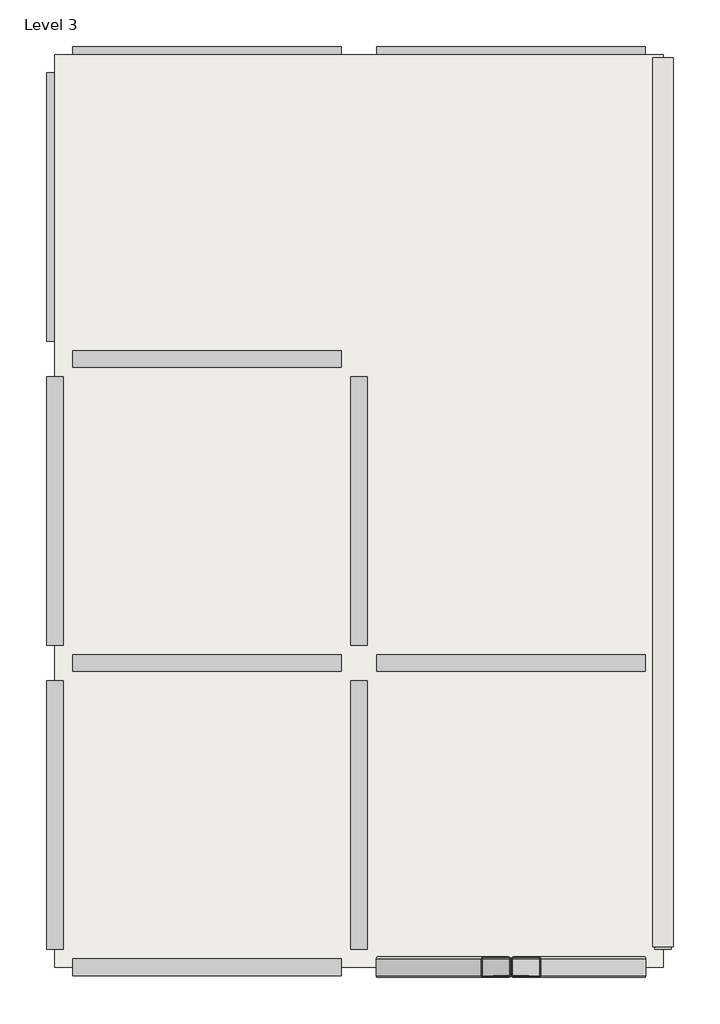
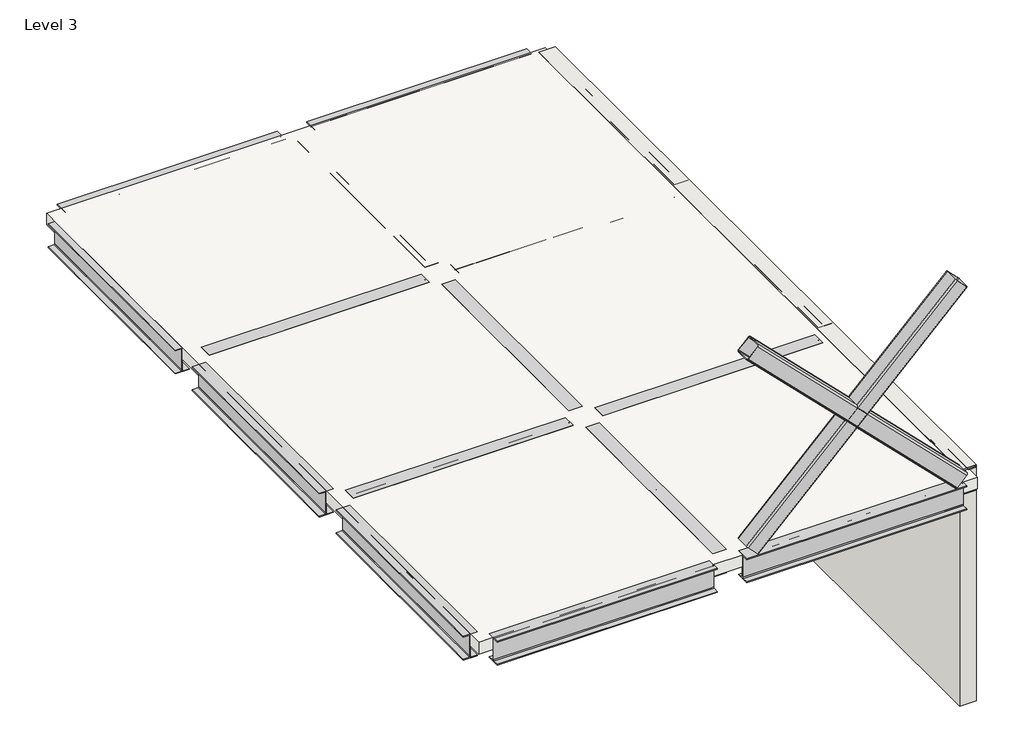
# One storey: 17 beams, 2 members, 1 slab, 1 wall.
"""IFC4 building model written with IfcOpenShell, lengths in millimetres."""

from ifc_helpers import new_model, si_unit, frame, origin, place, context, project, spatial, polyline, outline, extrude, transform, mapped, element, save
from components import ub_universal_beams_ub305x165x40_60ab2ee1, m_hss_square_hss203_2x203_2x9_5_07d005dd

model = new_model("IFC4")

# Units and contexts
model_context = context("Model", 3, world=origin())
ifc_project = project(units=[si_unit("LENGTHUNIT", "METRE", prefix="MILLI")], contexts=[model_context])

# Site, building, storey
site = spatial("IfcSite", under=ifc_project)
building = spatial("IfcBuilding", under=site)
storey = spatial("IfcBuildingStorey", under=building, Name="Level 3", Elevation=6000.0)

# Beams
placement = place(None, origin())
ub_universal_beams_ub305x165x40_shape = ub_universal_beams_ub305x165x40_60ab2ee1(model_context)
element("IfcBeam", 1, ObjectType="UB-Universal Beams : UB305x165x40", at=placement, inside=storey, context=model_context, shape_type="MappedRepresentation", body=[
    mapped(ub_universal_beams_ub305x165x40_shape, transform((18435.1404262, -6314.7314166, 5848.3), x_axis=(-1.0, 0.0, 0.0), y_axis=(0.0, -1.0, 0.0), z_axis=(0.0, 0.0, 1.0))),
])
element("IfcBeam", 2, ObjectType="UB-Universal Beams : UB305x165x40", at=placement, inside=storey, context=model_context, shape_type="MappedRepresentation", body=[
    mapped(ub_universal_beams_ub305x165x40_shape, transform((15435.1404262, -6314.7314166, 5848.3), x_axis=(-1.0, 0.0, 0.0), y_axis=(0.0, -1.0, 0.0), z_axis=(0.0, 0.0, 1.0))),
])
element("IfcBeam", 3, ObjectType="UB-Universal Beams : UB305x165x40", at=placement, inside=storey, context=model_context, shape_type="MappedRepresentation", body=[
    mapped(ub_universal_beams_ub305x165x40_shape, transform((13935.1404262, -4814.7314166, 5848.3), x_axis=(0.0, 1.0, 0.0), y_axis=(-1.0, 0.0, 0.0), z_axis=(0.0, 0.0, 1.0))),
])
element("IfcBeam", 4, ObjectType="UB-Universal Beams : UB305x165x40", at=placement, inside=storey, context=model_context, shape_type="MappedRepresentation", body=[
    mapped(ub_universal_beams_ub305x165x40_shape, transform((13935.1404262, -1814.7314166, 5848.3), x_axis=(0.0, 1.0, 0.0), y_axis=(-1.0, 0.0, 0.0), z_axis=(0.0, 0.0, 1.0))),
])
element("IfcBeam", 5, ObjectType="UB-Universal Beams : UB305x165x40", at=placement, inside=storey, context=model_context, shape_type="MappedRepresentation", body=[
    mapped(ub_universal_beams_ub305x165x40_shape, transform((13935.1404262, 1185.2685834, 5848.3), x_axis=(0.0, 1.0, 0.0), y_axis=(-1.0, 0.0, 0.0), z_axis=(0.0, 0.0, 1.0))),
])
element("IfcBeam", 6, ObjectType="UB-Universal Beams : UB305x165x40", at=placement, inside=storey, context=model_context, shape_type="MappedRepresentation", body=[
    mapped(ub_universal_beams_ub305x165x40_shape, transform((18435.1404262, -3314.7314166, 5848.3), x_axis=(-1.0, 0.0, 0.0), y_axis=(0.0, -1.0, 0.0), z_axis=(0.0, 0.0, 1.0))),
])
element("IfcBeam", 7, ObjectType="UB-Universal Beams : UB305x165x40", at=placement, inside=storey, context=model_context, shape_type="MappedRepresentation", body=[
    mapped(ub_universal_beams_ub305x165x40_shape, transform((15435.1404262, -3314.7314166, 5848.3), x_axis=(-1.0, 0.0, 0.0), y_axis=(0.0, -1.0, 0.0), z_axis=(0.0, 0.0, 1.0))),
])
element("IfcBeam", 8, ObjectType="UB-Universal Beams : UB305x165x40", at=placement, inside=storey, context=model_context, shape_type="MappedRepresentation", body=[
    mapped(ub_universal_beams_ub305x165x40_shape, transform((18435.1404262, -314.7314166, 5848.3), x_axis=(-1.0, 0.0, 0.0), y_axis=(0.0, -1.0, 0.0), z_axis=(0.0, 0.0, 1.0))),
])
element("IfcBeam", 9, ObjectType="UB-Universal Beams : UB305x165x40", at=placement, inside=storey, context=model_context, shape_type="MappedRepresentation", body=[
    mapped(ub_universal_beams_ub305x165x40_shape, transform((15435.1404262, -314.7314166, 5848.3), x_axis=(-1.0, 0.0, 0.0), y_axis=(0.0, -1.0, 0.0), z_axis=(0.0, 0.0, 1.0))),
])
element("IfcBeam", 10, ObjectType="UB-Universal Beams : UB305x165x40", at=placement, inside=storey, context=model_context, shape_type="MappedRepresentation", body=[
    mapped(ub_universal_beams_ub305x165x40_shape, transform((18435.1404262, 2685.2685834, 5848.3), x_axis=(-1.0, 0.0, 0.0), y_axis=(0.0, -1.0, 0.0), z_axis=(0.0, 0.0, 1.0))),
])
element("IfcBeam", 11, ObjectType="UB-Universal Beams : UB305x165x40", at=placement, inside=storey, context=model_context, shape_type="MappedRepresentation", body=[
    mapped(ub_universal_beams_ub305x165x40_shape, transform((15435.1404262, 2685.2685834, 5848.3), x_axis=(-1.0, 0.0, 0.0), y_axis=(0.0, -1.0, 0.0), z_axis=(0.0, 0.0, 1.0))),
])
element("IfcBeam", 12, ObjectType="UB-Universal Beams : UB305x165x40", at=placement, inside=storey, context=model_context, shape_type="MappedRepresentation", body=[
    mapped(ub_universal_beams_ub305x165x40_shape, transform((16935.1404262, -4814.7314166, 5848.3), x_axis=(0.0, 1.0, 0.0), y_axis=(-1.0, 0.0, 0.0), z_axis=(0.0, 0.0, 1.0))),
])
element("IfcBeam", 13, ObjectType="UB-Universal Beams : UB305x165x40", at=placement, inside=storey, context=model_context, shape_type="MappedRepresentation", body=[
    mapped(ub_universal_beams_ub305x165x40_shape, transform((16935.1404262, -1814.7314166, 5848.3), x_axis=(0.0, 1.0, 0.0), y_axis=(-1.0, 0.0, 0.0), z_axis=(0.0, 0.0, 1.0))),
])
element("IfcBeam", 14, ObjectType="UB-Universal Beams : UB305x165x40", at=placement, inside=storey, context=model_context, shape_type="MappedRepresentation", body=[
    mapped(ub_universal_beams_ub305x165x40_shape, transform((16935.1404262, 1185.2685834, 5848.3), x_axis=(0.0, 1.0, 0.0), y_axis=(-1.0, 0.0, 0.0), z_axis=(0.0, 0.0, 1.0))),
])
element("IfcBeam", 15, ObjectType="UB-Universal Beams : UB305x165x40", at=placement, inside=storey, context=model_context, shape_type="MappedRepresentation", body=[
    mapped(ub_universal_beams_ub305x165x40_shape, transform((19935.1404262, -1814.7314166, 5848.3), x_axis=(0.0, 1.0, 0.0), y_axis=(-1.0, 0.0, 0.0), z_axis=(0.0, 0.0, 1.0))),
])
element("IfcBeam", 16, ObjectType="UB-Universal Beams : UB305x165x40", at=placement, inside=storey, context=model_context, shape_type="MappedRepresentation", body=[
    mapped(ub_universal_beams_ub305x165x40_shape, transform((19935.1404262, 1185.2685834, 5848.3), x_axis=(0.0, 1.0, 0.0), y_axis=(-1.0, 0.0, 0.0), z_axis=(0.0, 0.0, 1.0))),
])
element("IfcBeam", 17, ObjectType="UB-Universal Beams : beam", at=placement, inside=storey, context=model_context, shape_type="MappedRepresentation", body=[
    mapped(ub_universal_beams_ub305x165x40_shape, transform((19935.1404262, -4814.7314166, 5848.3), x_axis=(0.0, 1.0, 0.0), y_axis=(-1.0, 0.0, 0.0), z_axis=(0.0, 0.0, 1.0))),
])

# Members
m_hss_square_hss203_2x203_2x9_5_shape = m_hss_square_hss203_2x203_2x9_5_07d005dd(model_context)
element("IfcMember", 18, ObjectType="M_HSS Square : HSS203.2X203.2X9.5", at=placement, inside=storey, context=model_context, shape_type="MappedRepresentation", body=[
    mapped(m_hss_square_hss203_2x203_2x9_5_shape, transform((18435.1404262, -6314.7314166, 7348.3), x_axis=(-0.7071067811865478, 0.0, 0.7071067811865476), y_axis=(0.0, -1.0000000000000002, 0.0), z_axis=(0.7071067811865476, 0.0, 0.7071067811865478))),
])
element("IfcMember", 19, ObjectType="M_HSS Square : HSS203.2X203.2X9.5", at=placement, inside=storey, context=model_context, shape_type="MappedRepresentation", body=[
    mapped(m_hss_square_hss203_2x203_2x9_5_shape, transform((18435.1404262, -6314.7314166, 7348.3), x_axis=(-0.7071067811865478, 0.0, -0.7071067811865475), y_axis=(0.0, -1.0000000000000002, 0.0), z_axis=(-0.7071067811865475, 0.0, 0.7071067811865478))),
])

# Slab
element("IfcSlab", 20, ObjectType="150mm Foundation Slab", at=placement, inside=storey, context=model_context, shape_type="SweptSolid", body=[
    extrude(outline(polyline([(13935.1404262, -6314.7314166), (13935.1404262, 2685.2685834), (19935.1404262, 2685.2685834), (19935.1404262, -6314.7314166), (13935.1404262, -6314.7314166)])), frame((0.0, 0.0, 5850.0), z_axis=(0.0, 0.0, 1.0), x_axis=(1.0, 0.0, 0.0)), (0.0, 0.0, 1.0), 150.0),
])

# Wall
element("IfcWall", 21, ObjectType="Generic - 200mm", at=placement, inside=storey, context=model_context, shape_type="SweptSolid", body=[
    extrude(outline(polyline([(19835.1404262, -6114.7314166), (19835.1404262, 2655.9792615), (20035.1404262, 2655.9792615), (20035.1404262, -6114.7314166), (19835.1404262, -6114.7314166)])), frame((0.0, 0.0, 3000.0), z_axis=(0.0, 0.0, 1.0), x_axis=(1.0, 0.0, 0.0)), (0.0, 0.0, 1.0), 3000.0),
])

save(model, "model.ifc")

# Revit data of these elements
# Type "UB-Universal Beams : UB305x165x40"
#   Section Name Key = "UB305X165X40"
#   Width = 16.5 cm
#   Web Thickness = 0.6 cm
#   Web Fillet = 0.89 cm
#   Warping Constant = 164000.0 cm⁶
#   Torsional Moment of Inertia = 14.70 cm⁴
#   Section Area = 51.3 cm²
#   Plastic Modulus weak axis = 142.0 cm³
#   Plastic Modulus strong axis = 623.0 cm³
#   Nominal Weight = 40.2999 kgf/m
#   Moment of Inertia weak axis = 764.00 cm⁴
#   Moment of Inertia strong axis = 8503.00 cm⁴
#   Height = 30.34 cm
#   Flange Thickness = 1.02 cm
#   Elastic Modulus weak axis = 92.6 cm³
#   Elastic Modulus strong axis = 560.0 cm³
#   Centroid Vertical = 15.17 cm
#   Centroid Horizontal = 8.25 cm
#   Bolt Spacing = 9.0 cm
#   Length [instance default] = 1.5 m
#   Structural Material [instance default] = Metal - Steel 43-275
#   Type Comments = ""
#   Assembly Code = ""
# Type "UB-Universal Beams : beam"
#   Section Name Key = "UB305X165X40"
#   Width = 16.5 cm
#   Web Thickness = 0.6 cm
#   Web Fillet = 0.89 cm
#   Warping Constant = 164000.0 cm⁶
#   Torsional Moment of Inertia = 14.70 cm⁴
#   Section Area = 51.3 cm²
#   Plastic Modulus weak axis = 142.0 cm³
#   Plastic Modulus strong axis = 623.0 cm³
#   Nominal Weight = 40.2999 kgf/m
#   Moment of Inertia weak axis = 764.00 cm⁴
#   Moment of Inertia strong axis = 8503.00 cm⁴
#   Height = 30.34 cm
#   Flange Thickness = 1.02 cm
#   Elastic Modulus weak axis = 92.6 cm³
#   Elastic Modulus strong axis = 560.0 cm³
#   Centroid Vertical = 15.17 cm
#   Centroid Horizontal = 8.25 cm
#   Bolt Spacing = 9.0 cm
#   Length [instance default] = 1.5 m
#   Structural Material [instance default] = Metal - Steel 43-275
#   Type Comments = ""
#   Assembly Code = ""
# Type "M_HSS Square : HSS203.2X203.2X9.5"
#   Section Name Key = "HSS 8X8X3/8"
#   Width = 20.3 cm
#   Wall Nominal Thickness = 0.953 cm
#   Wall Design Thickness = 0.886 cm
#   Torsional Moment of Inertia = 6660.00 cm⁴
#   Torsional Modulus = 10930171.7 cm³
#   Section Area = 67.1 cm²
#   Plastic Modulus weak axis = 482.0 cm³
#   Plastic Modulus strong axis = 482.0 cm³
#   Outer Fillet = 1.906 cm
#   Nominal Weight = 55.9998 kgf/m
#   Moment of Inertia weak axis = 4160.00 cm⁴
#   Moment of Inertia strong axis = 4160.00 cm⁴
#   Length [instance default] = 1.524 m
#   Inner Fillet = 0.953 cm
#   Height = 20.3 cm
#   Elastic Modulus weak axis = 408.0 cm³
#   Elastic Modulus strong axis = 408.0 cm³
#   Centroid Vertical = 10.15 cm
#   Centroid Horizontal = 10.15 cm
#   Structural Material [instance default] = Steel, 45-345
# Type "150mm Foundation Slab"
#   Layers, outside or top first: 0.15 m "Concrete, Cast-in-Place gray" (function 1)
# Type "Generic - 200mm"
#   Layers, outside or top first: 0.2 m no material (function 1)
# Elements 1, 2, 3, 4, 5, 6, 7, 8, 9, 10, 11, 12, 13, 14, 15, 16 (IfcBeam, "UB-Universal Beams : UB305x165x40")
#   Structural Material = Metal - Steel 43-275
#   Phase Created = New Construction
#   Materials on its faces: "Metal - Steel 43-275"
# Element 17 (IfcBeam, "UB-Universal Beams : beam")
#   Structural Material = Metal - Steel 43-275
#   Phase Created = New Construction
#   Materials on its faces: "Metal - Steel 43-275"
# Elements 18, 19 (IfcMember, "M_HSS Square : HSS203.2X203.2X9.5")
#   Comments = ""
#   Structural Material = Metal - Steel 43-275
#   Phase Created = New Construction
#   Materials on its faces: "Metal - Steel 43-275"
# Element 20 (IfcSlab, "150mm Foundation Slab")
#   built-in parameter 1001955 = 3.14159 (stored number, unit not read)
#   Height Offset From Level = 0 m
#   built-in parameter 1001954 = 1
#   Phase Created = New Construction
#   Materials on its faces: "Concrete, Cast-in-Place gray"
# Element 21 (IfcWall, "Generic - 200mm")
#   Comments = ""
#   built-in parameter 1001111 = -3 m
#   Top Offset = 0 m
#   Base Offset = -3 m
#   wall height = 3 m
#   Phase Created = New Construction
#   Base Constraint = Level 3
#   Top Constraint = Level 3
#   Materials on its faces: "Default Wall"
# Materials
#   "Metal - Steel 43-275": class "Metal", colour RGB 247 247 247, transparency 0, Cost = 0
#   "Steel, 45-345": class "Metal", colour RGB 247 247 247, transparency 0, Description = "Steel 345 MPa", Cost = 0
#   "Concrete, Cast-in-Place gray": class "Concrete", colour RGB 192 192 192, transparency 0, Description = "Cast-in-place concrete", Cost = 0
#   "Default Wall": colour RGB 128 128 128, transparency 0, Cost = 0
